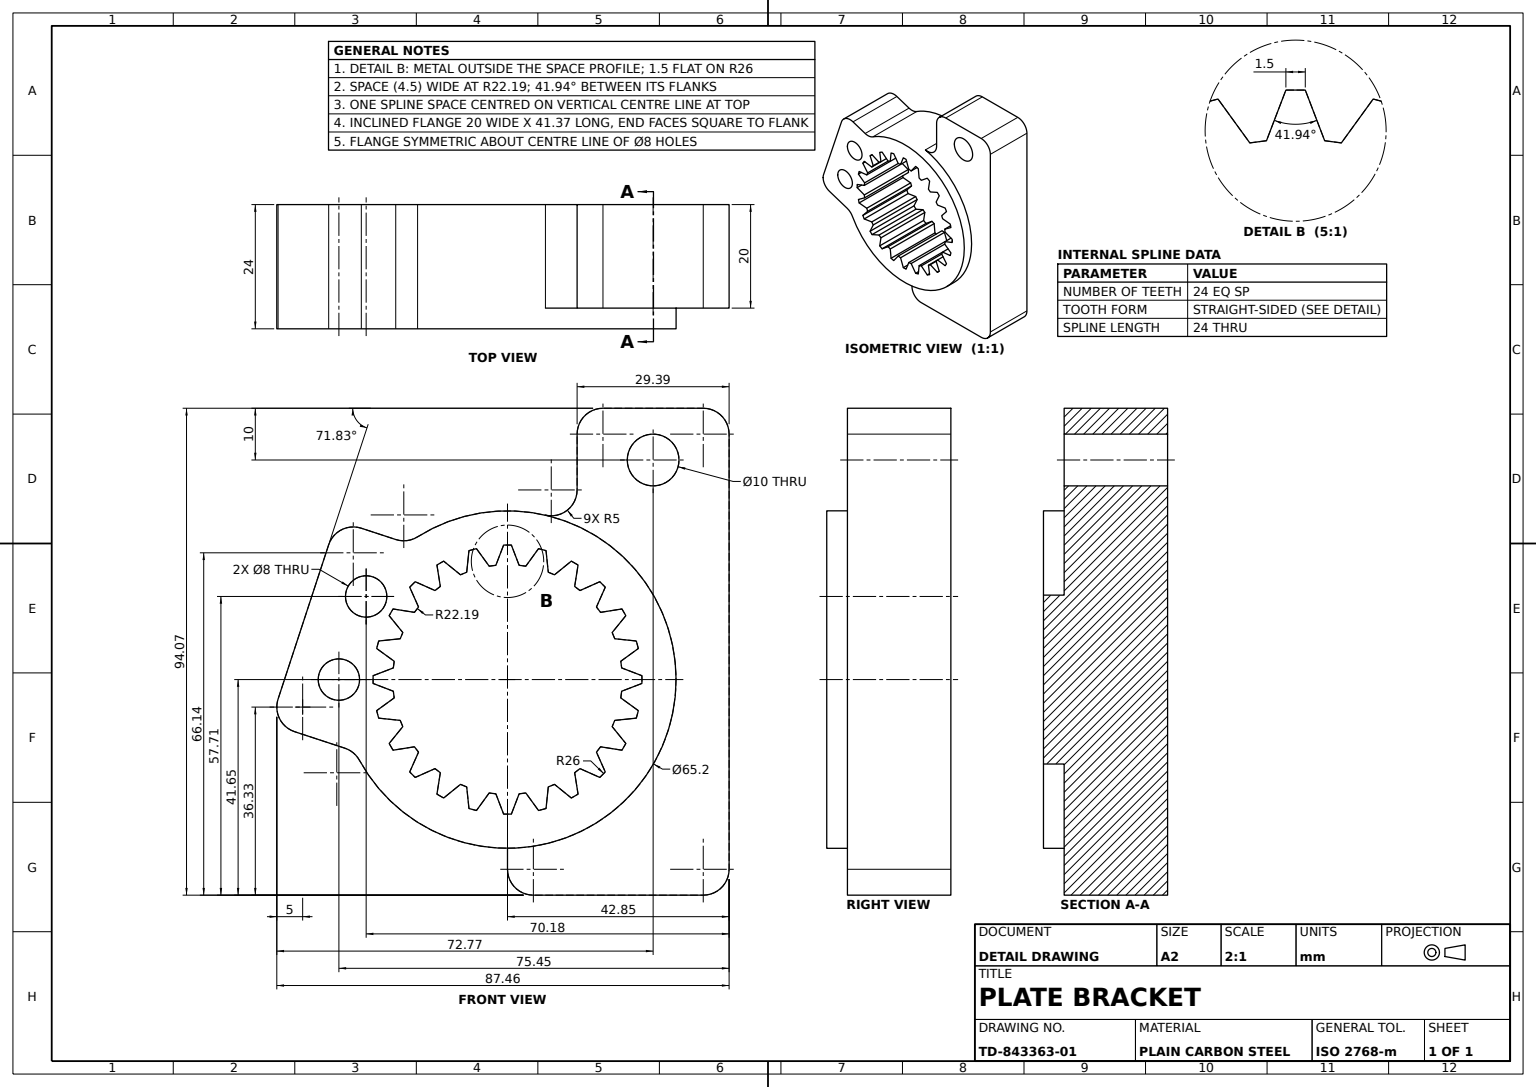
from build123d import *

# Parameters (mm, degrees)
MOUNTING_PLATE_DEPTH          = 20
SKETCH1_7_R                   = 32.6
SPLINE_HUB_BOSS_DEPTH         = 24
FLANGE_START                  = -24
FLANGE_BOSS_DEPTH             = 24
SKETCH3_4_R                   = 4
FLANGE_MOUNTING_HOLE_DEPTH    = 24
PLATE_HOLE_SKETCH_R           = 5
PLATE_MOUNTING_HOLE_DEPTH     = 24
INTERNAL_SPLINE_CUT_24T_DEPTH = 24
EDGE_FILLETS_R5_R             = 5


with BuildPart() as part:
    # Bracket Profile Sketch → Mounting Plate (new body)
    with BuildSketch(Plane.XY):
        with BuildLine():
            ThreePointArc((32.6, 0), (23.051681067, -23.051681067), (0, -32.6))
            Line((0, -32.6), (0, -41.65))
            Line((0, -41.65), (42.85, -41.65))
            Line((42.85, -41.65), (42.85, 52.42))
            Line((42.85, 52.42), (13.46, 52.42))
            Line((13.46, 52.42), (13.46, 29.691554355))
            ThreePointArc((13.46, 29.691554355), (27.400328465, 17.663012201), (32.6, 0))
        make_face()
    extrude(amount=MOUNTING_PLATE_DEPTH)

    # Sketch1_7 → Spline Hub Boss (add)
    with BuildSketch(Plane.XY):
        with Locations(Location((0, 0, 0), (0, 0, 270))):
            Circle(SKETCH1_7_R)
    extrude(amount=SPLINE_HUB_BOSS_DEPTH)

    # Flange and Hole Sketch → Flange Boss (add)
    with BuildSketch(Plane.XY.offset(24).offset(FLANGE_START)):
        with BuildLine():
            Line((-33.01607204, 30.800569947), (-45.916657839, -8.506576808))
            Line((-45.916657839, -8.506576808), (-29.489019594, -13.89811942))
            ThreePointArc((-29.489019594, -13.89811942), (-31.315952081, -9.059312625), (-32.354601227, -3.992465334))
            ThreePointArc((-32.354601227, -3.992465334), (-36.6, 0), (-32.354601227, 3.992465334))
            ThreePointArc((-32.354601227, 3.992465334), (-31.45055914, 8.580345552), (-29.899432156, 12.991687986))
            ThreePointArc((-29.899432156, 12.991687986), (-30.778793233, 18.08359035), (-25.90281989, 19.79403753))
            ThreePointArc((-25.90281989, 19.79403753), (-22.821560181, 23.279527292), (-19.275545993, 26.290936208))
            Line((-19.275545993, 26.290936208), (-33.01607204, 30.800569947))
        make_face()
    extrude(amount=FLANGE_BOSS_DEPTH)

    # Sketch3_4 → Flange Mounting Hole (cut)
    with BuildSketch(Plane.XY.offset(24).offset(FLANGE_START)):
        with Locations((-32.6, 0)):
            Circle(SKETCH3_4_R)
        with Locations((-27.33, 16.057306748)):
            Circle(SKETCH3_4_R)
    extrude(amount=FLANGE_MOUNTING_HOLE_DEPTH, mode=Mode.SUBTRACT)

    # Plate Hole Sketch → Plate Mounting Hole (cut)
    with BuildSketch(Plane.XY.offset(20)):
        with Locations((28.16, 42.42)):
            Circle(PLATE_HOLE_SKETCH_R)
    extrude(amount=-PLATE_MOUNTING_HOLE_DEPTH, mode=Mode.SUBTRACT)

    # Internal Spline Profile 24T → Internal Spline Cut 24T (cut)
    with BuildSketch(Plane.XY.offset(24)):
        with BuildLine():
            Line((-6.002050495, -25.297734876), (-3.540261306, -21.905767503))
            ThreePointArc((-3.540261306, -21.905767503), (-2.896376205, -22.000161474), (-2.25, -22.075633626))
            Line((-2.25, -22.075633626), (-0.75, -25.989180441))
            ThreePointArc((-0.75, -25.989180441), (0, -26), (0.75, -25.989180441))
            Line((0.75, -25.989180441), (2.25, -22.075633626))
            ThreePointArc((2.25, -22.075633626), (2.896376205, -22.000161474), (3.540261306, -21.905767503))
            Line((3.540261306, -21.905767503), (6.002050495, -25.297734876))
            ThreePointArc((6.002050495, -25.297734876), (6.729295173, -25.114071484), (7.450939234, -24.909506308))
            Line((7.450939234, -24.909506308), (7.886927524, -20.7410818))
            ThreePointArc((7.886927524, -20.7410818), (8.491745364, -20.500886826), (9.089259655, -20.243059525))
            Line((9.089259655, -20.243059525), (12.345071168, -22.882290486))
            ThreePointArc((12.345071168, -22.882290486), (13, -22.516660498), (13.644109273, -22.132290486))
            Line((13.644109273, -22.132290486), (12.986373972, -17.993059525))
            ThreePointArc((12.986373972, -17.993059525), (13.50841611, -17.604510621), (14.018839978, -17.200820494))
            Line((14.018839978, -17.200820494), (17.846795641, -18.907455813))
            ThreePointArc((17.846795641, -18.907455813), (18.384776311, -18.384776311), (18.907455813, -17.846795641))
            Line((18.907455813, -17.846795641), (17.200820494, -14.018839978))
            ThreePointArc((17.200820494, -14.018839978), (17.604510621, -13.50841611), (17.993059525, -12.986373972))
            Line((17.993059525, -12.986373972), (22.132290486, -13.644109273))
            ThreePointArc((22.132290486, -13.644109273), (22.516660498, -13), (22.882290486, -12.345071168))
            Line((22.882290486, -12.345071168), (20.243059525, -9.089259655))
            ThreePointArc((20.243059525, -9.089259655), (20.500886826, -8.491745364), (20.7410818, -7.886927524))
            Line((20.7410818, -7.886927524), (24.909506308, -7.450939234))
            ThreePointArc((24.909506308, -7.450939234), (25.114071484, -6.729295173), (25.297734876, -6.002050495))
            Line((25.297734876, -6.002050495), (21.905767503, -3.540261306))
            ThreePointArc((21.905767503, -3.540261306), (22.000161474, -2.896376205), (22.075633626, -2.25))
            Line((22.075633626, -2.25), (25.989180441, -0.75))
            ThreePointArc((25.989180441, -0.75), (25.99729497, -0.375039019), (26, 0))
            ThreePointArc((26, 0), (25.99729497, 0.375039019), (25.989180441, 0.75))
            Line((25.989180441, 0.75), (22.075633626, 2.25))
            ThreePointArc((22.075633626, 2.25), (22.000161474, 2.896376205), (21.905767503, 3.540261306))
            Line((21.905767503, 3.540261306), (25.297734876, 6.002050495))
            ThreePointArc((25.297734876, 6.002050495), (25.114071484, 6.729295173), (24.909506308, 7.450939234))
            Line((24.909506308, 7.450939234), (20.7410818, 7.886927524))
            ThreePointArc((20.7410818, 7.886927524), (20.500886826, 8.491745364), (20.243059525, 9.089259655))
            Line((20.243059525, 9.089259655), (22.882290486, 12.345071168))
            ThreePointArc((22.882290486, 12.345071168), (22.516660498, 13), (22.132290486, 13.644109273))
            Line((22.132290486, 13.644109273), (17.993059525, 12.986373972))
            ThreePointArc((17.993059525, 12.986373972), (17.604510621, 13.50841611), (17.200820494, 14.018839978))
            Line((17.200820494, 14.018839978), (18.907455813, 17.846795641))
            ThreePointArc((18.907455813, 17.846795641), (18.384776311, 18.384776311), (17.846795641, 18.907455813))
            Line((17.846795641, 18.907455813), (14.018839978, 17.200820494))
            ThreePointArc((14.018839978, 17.200820494), (13.50841611, 17.604510621), (12.986373972, 17.993059525))
            Line((12.986373972, 17.993059525), (13.644109273, 22.132290486))
            ThreePointArc((13.644109273, 22.132290486), (13, 22.516660498), (12.345071168, 22.882290486))
            Line((12.345071168, 22.882290486), (9.089259655, 20.243059525))
            ThreePointArc((9.089259655, 20.243059525), (8.491745364, 20.500886826), (7.886927524, 20.7410818))
            Line((7.886927524, 20.7410818), (7.450939234, 24.909506308))
            ThreePointArc((7.450939234, 24.909506308), (6.729295173, 25.114071484), (6.002050495, 25.297734876))
            Line((6.002050495, 25.297734876), (3.540261306, 21.905767503))
            ThreePointArc((3.540261306, 21.905767503), (2.896376205, 22.000161474), (2.25, 22.075633626))
            Line((2.25, 22.075633626), (0.75, 25.989180441))
            ThreePointArc((0.75, 25.989180441), (0, 26), (-0.75, 25.989180441))
            Line((-0.75, 25.989180441), (-2.25, 22.075633626))
            ThreePointArc((-2.25, 22.075633626), (-2.896376205, 22.000161474), (-3.540261306, 21.905767503))
            Line((-3.540261306, 21.905767503), (-6.002050495, 25.297734876))
            ThreePointArc((-6.002050495, 25.297734876), (-6.729295173, 25.114071484), (-7.450939234, 24.909506308))
            Line((-7.450939234, 24.909506308), (-7.886927524, 20.7410818))
            ThreePointArc((-7.886927524, 20.7410818), (-8.491745364, 20.500886826), (-9.089259655, 20.243059525))
            Line((-9.089259655, 20.243059525), (-12.345071168, 22.882290486))
            ThreePointArc((-12.345071168, 22.882290486), (-13, 22.516660498), (-13.644109273, 22.132290486))
            Line((-13.644109273, 22.132290486), (-12.986373972, 17.993059525))
            ThreePointArc((-12.986373972, 17.993059525), (-13.50841611, 17.604510621), (-14.018839978, 17.200820494))
            Line((-14.018839978, 17.200820494), (-17.846795641, 18.907455813))
            ThreePointArc((-17.846795641, 18.907455813), (-18.384776311, 18.384776311), (-18.907455813, 17.846795641))
            Line((-18.907455813, 17.846795641), (-17.200820494, 14.018839978))
            ThreePointArc((-17.200820494, 14.018839978), (-17.604510621, 13.50841611), (-17.993059525, 12.986373972))
            Line((-17.993059525, 12.986373972), (-22.132290486, 13.644109273))
            ThreePointArc((-22.132290486, 13.644109273), (-22.516660498, 13), (-22.882290486, 12.345071168))
            Line((-22.882290486, 12.345071168), (-20.243059525, 9.089259655))
            ThreePointArc((-20.243059525, 9.089259655), (-20.500886826, 8.491745364), (-20.7410818, 7.886927524))
            Line((-20.7410818, 7.886927524), (-24.909506308, 7.450939234))
            ThreePointArc((-24.909506308, 7.450939234), (-25.114071484, 6.729295173), (-25.297734876, 6.002050495))
            Line((-25.297734876, 6.002050495), (-21.905767503, 3.540261306))
            ThreePointArc((-21.905767503, 3.540261306), (-22.000161474, 2.896376205), (-22.075633626, 2.25))
            Line((-22.075633626, 2.25), (-25.989180441, 0.75))
            ThreePointArc((-25.989180441, 0.75), (-26, 0), (-25.989180441, -0.75))
            Line((-25.989180441, -0.75), (-22.075633626, -2.25))
            ThreePointArc((-22.075633626, -2.25), (-22.000161474, -2.896376205), (-21.905767503, -3.540261306))
            Line((-21.905767503, -3.540261306), (-25.297734876, -6.002050495))
            ThreePointArc((-25.297734876, -6.002050495), (-25.114071484, -6.729295173), (-24.909506308, -7.450939234))
            Line((-24.909506308, -7.450939234), (-20.7410818, -7.886927524))
            ThreePointArc((-20.7410818, -7.886927524), (-20.500886826, -8.491745364), (-20.243059525, -9.089259655))
            Line((-20.243059525, -9.089259655), (-22.882290486, -12.345071168))
            ThreePointArc((-22.882290486, -12.345071168), (-22.516660498, -13), (-22.132290486, -13.644109273))
            Line((-22.132290486, -13.644109273), (-17.993059525, -12.986373972))
            ThreePointArc((-17.993059525, -12.986373972), (-17.604510621, -13.50841611), (-17.200820494, -14.018839978))
            Line((-17.200820494, -14.018839978), (-18.907455813, -17.846795641))
            ThreePointArc((-18.907455813, -17.846795641), (-18.384776311, -18.384776311), (-17.846795641, -18.907455813))
            Line((-17.846795641, -18.907455813), (-14.018839978, -17.200820494))
            ThreePointArc((-14.018839978, -17.200820494), (-13.50841611, -17.604510621), (-12.986373972, -17.993059525))
            Line((-12.986373972, -17.993059525), (-13.644109273, -22.132290486))
            ThreePointArc((-13.644109273, -22.132290486), (-13, -22.516660498), (-12.345071168, -22.882290486))
            Line((-12.345071168, -22.882290486), (-9.089259655, -20.243059525))
            ThreePointArc((-9.089259655, -20.243059525), (-8.491745364, -20.500886826), (-7.886927524, -20.7410818))
            Line((-7.886927524, -20.7410818), (-7.450939234, -24.909506308))
            ThreePointArc((-7.450939234, -24.909506308), (-6.729295173, -25.114071484), (-6.002050495, -25.297734876))
        make_face()
    extrude(amount=-INTERNAL_SPLINE_CUT_24T_DEPTH, mode=Mode.SUBTRACT)

    # Edge Fillets R5
    edge_fillets_r5_edges = [part.edges().sort_by_distance(p)[0] for p in [
        (13.46, 29.691554355, 10),
        (13.46, 52.42, 10),
        (42.85, 52.42, 10),
        (42.85, -41.65, 10),
        (0, -41.65, 10),
        (-29.489019594, -13.89811942, 12),
        (-45.916657839, -8.506576808, 12),
        (-33.01607204, 30.800569947, 12),
        (-19.275545993, 26.290936208, 12),
    ]]
    fillet(edge_fillets_r5_edges, radius=EDGE_FILLETS_R5_R)


solid = part.part
